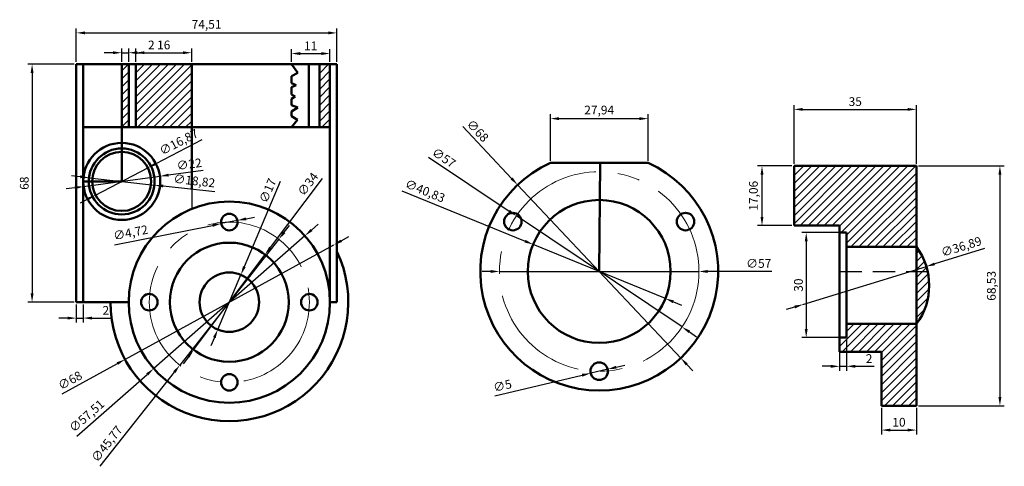
# Model space of a CAD drawing. Units: millimetres. Extents: x 1194 to 1920, y 1729 to 2086.
# Tile 2 of 5: x 1194 to 1475, y 1948 to 2076. Entities that reach past the tile are written whole.
import ezdxf

# ---------------------------------------------------------------- set-up
doc = ezdxf.new("R2010")
doc.units = ezdxf.units.MM
doc.linetypes.add('CENTER', pattern=[50.8, 31.75, -6.35, 6.35, -6.35])
doc.linetypes.add('HIDDEN', pattern=[9.525, 6.35, -3.175])
for name, color, linetype, lineweight in [('M-CNTR', 1, 'CENTER', 18), ('M-DIMS', 2, 'Continuous', 25), ('M-HATC', 8, 'Continuous', 18), ('M-HIDN', 4, 'HIDDEN', 25), ('M-OUTL', 7, 'Continuous', 50)]:
    doc.layers.add(name, color=color, linetype=linetype, lineweight=lineweight)
doc.styles.get("Standard").update_dxf_attribs({"font": 'arial.ttf'})
doc.dimstyles.new('ISO-25', dxfattribs={"dimtxt": 2.5, "dimasz": 2.5, "dimexe": 1.25, "dimexo": 0.625, "dimtad": 1, "dimtxsty": 'Standard', "dimcen": 2.5, "dimadec": 0, "dimazin": 0, "dimtfac": 1, "dimtmove": 0, "dimatfit": 3, "dimfxl": 1, "dimarcsym": 0})

# ---------------------------------------------------------------- blocks, each defined once
blk = doc.blocks.new('*U1')
blk.add_circle((0, 0), 2.36)
blk = doc.blocks.new('*U2')
at = {"layer": 'M-OUTL', "color": 0, "linetype": 'ByBlock', "lineweight": -2, "transparency": 16777216}
blk.add_blockref('*U1', (1253.67, 2017.83), dxfattribs=at)
for p, rotation in [((1230.79, 1994.94), 90), ((1276.56, 1994.94), 270), ((1253.67, 1972.06), 180)]:
    blk.add_blockref('*U1', p, dxfattribs=dict(at, rotation=rotation))
blk = doc.blocks.new('*U3')
blk.add_circle((0, 0), 2.5)
blk = doc.blocks.new('*U4')
at = {"layer": 'M-OUTL', "color": 0, "linetype": 'ByBlock', "lineweight": -2, "transparency": 16777216}
for p, rotation in [((1334.73, 2017.97), 240), ((1384.09, 2017.97), 119.9999999999999)]:
    blk.add_blockref('*U3', p, dxfattribs=dict(at, rotation=rotation))
blk.add_blockref('*U3', (1359.41, 1975.22), dxfattribs=at)
blk = doc.blocks.new('*D13')
at = {"layer": 'Defpoints', "color": 0, "transparency": 16777216}
for p in [(1283.49, 2011.28), (1223.86, 1978.6)]:
    blk.add_point(p, dxfattribs=at)
at = {"layer": 'M-DIMS', "color": 0, "lineweight": -2, "transparency": 16777216}
for p, q in [((1285.68, 2012.49), (1287.87, 2013.69)), ((1283.49, 2011.28), (1223.86, 1978.6)), ((1205.92, 1968.78), (1221.66, 1977.4))]:
    blk.add_line(p, q, dxfattribs=at)
at = {"layer": 'M-DIMS', "color": 0, "transparency": 16777216}
for points in [[(1285.48, 2012.85), (1285.88, 2012.12), (1283.49, 2011.28)], [(1221.46, 1977.77), (1221.86, 1977.04), (1223.86, 1978.6)]]:
    blk.add_solid(points, dxfattribs=at)
at = {"layer": 'M-DIMS', "color": 0, "transparency": 16777216, "insert": (1208.29, 1972.32), "char_height": 2.5, "attachment_point": 5, "rotation": 28.7233}
blk.add_mtext('∅68', dxfattribs=at)
blk = doc.blocks.new('*D14')
at = {"layer": 'Defpoints', "color": 0, "transparency": 16777216}
for p in [(1275.28, 2013.91), (1232.06, 1975.97)]:
    blk.add_point(p, dxfattribs=at)
at = {"layer": 'M-DIMS', "color": 0, "lineweight": -2, "transparency": 16777216}
for p, q in [((1277.16, 2015.56), (1279.04, 2017.21)), ((1275.28, 2013.91), (1232.06, 1975.97)), ((1210.06, 1956.65), (1230.19, 1974.33))]:
    blk.add_line(p, q, dxfattribs=at)
at = {"layer": 'M-DIMS', "color": 0, "transparency": 16777216}
for points in [[(1276.88, 2015.88), (1277.43, 2015.25), (1275.28, 2013.91)], [(1229.91, 1974.64), (1230.46, 1974.01), (1232.06, 1975.97)]]:
    blk.add_solid(points, dxfattribs=at)
at = {"layer": 'M-DIMS', "color": 0, "transparency": 16777216, "insert": (1213.11, 1962.22), "char_height": 2.5, "attachment_point": 5, "rotation": 41.2792}
blk.add_mtext('∅57,51', dxfattribs=at)
blk = doc.blocks.new('*D15')
at = {"layer": 'Defpoints', "color": 0, "transparency": 16777216}
for p in [(1267.82, 2012.93), (1239.52, 1976.96)]:
    blk.add_point(p, dxfattribs=at)
at = {"layer": 'M-DIMS', "color": 0, "lineweight": -2, "transparency": 16777216}
for p, q in [((1269.37, 2014.9), (1270.92, 2016.86)), ((1267.82, 2012.93), (1239.52, 1976.96)), ((1216.79, 1948.06), (1237.98, 1974.99))]:
    blk.add_line(p, q, dxfattribs=at)
at = {"layer": 'M-DIMS', "color": 0, "transparency": 16777216}
for points in [[(1269.04, 2015.15), (1269.7, 2014.64), (1267.82, 2012.93)], [(1237.65, 1975.25), (1238.3, 1974.73), (1239.52, 1976.96)]]:
    blk.add_solid(points, dxfattribs=at)
at = {"layer": 'M-DIMS', "color": 0, "transparency": 16777216, "insert": (1218.92, 1954.28), "char_height": 2.5, "attachment_point": 5, "rotation": 51.8058}
blk.add_mtext('∅45,77', dxfattribs=at)
blk = doc.blocks.new('*D16')
at = {"layer": 'Defpoints', "color": 0, "transparency": 16777216}
for p in [(1263.88, 2008.54), (1243.47, 1981.35)]:
    blk.add_point(p, dxfattribs=at)
at = {"layer": 'M-DIMS', "color": 0, "lineweight": -2, "transparency": 16777216}
for p, q in [((1280.22, 2030.3), (1265.38, 2010.54)), ((1243.47, 1981.35), (1263.88, 2008.54)), ((1241.96, 1979.35), (1240.46, 1977.35))]:
    blk.add_line(p, q, dxfattribs=at)
at = {"layer": 'M-DIMS', "color": 0, "transparency": 16777216}
for points in [[(1265.05, 2010.79), (1265.71, 2010.29), (1263.88, 2008.54)], [(1241.63, 1979.6), (1242.3, 1979.1), (1243.47, 1981.35)]]:
    blk.add_solid(points, dxfattribs=at)
at = {"layer": 'M-DIMS', "color": 0, "transparency": 16777216, "insert": (1276.38, 2028.47), "char_height": 2.5, "attachment_point": 5, "rotation": 53.1003}
blk.add_mtext('∅34', dxfattribs=at)
blk = doc.blocks.new('*D17')
at = {"layer": 'Defpoints', "color": 0, "transparency": 16777216}
for p in [(1256.98, 2002.77), (1250.36, 1987.11)]:
    blk.add_point(p, dxfattribs=at)
at = {"layer": 'M-DIMS', "color": 0, "lineweight": -2, "transparency": 16777216}
for p, q in [((1268.23, 2029.39), (1257.96, 2005.08)), ((1250.36, 1987.11), (1256.98, 2002.77)), ((1249.39, 1984.81), (1248.42, 1982.51))]:
    blk.add_line(p, q, dxfattribs=at)
at = {"layer": 'M-DIMS', "color": 0, "transparency": 16777216}
for points in [[(1257.57, 2005.24), (1258.34, 2004.91), (1256.98, 2002.77)], [(1249.01, 1984.97), (1249.77, 1984.65), (1250.36, 1987.11)]]:
    blk.add_solid(points, dxfattribs=at)
at = {"layer": 'M-DIMS', "color": 0, "transparency": 16777216, "insert": (1264.95, 2026.68), "char_height": 2.5, "attachment_point": 5, "rotation": 67.0856}
blk.add_mtext('∅17', dxfattribs=at)
blk = doc.blocks.new('*D18')
at = {"layer": 'Defpoints', "color": 0, "transparency": 16777216}
for p in [(1255.99, 2018.29), (1251.35, 2017.38)]:
    blk.add_point(p, dxfattribs=at)
at = {"layer": 'M-DIMS', "color": 0, "lineweight": -2, "transparency": 16777216}
for p, q in [((1255.99, 2018.29), (1251.35, 2017.38)), ((1258.44, 2018.77), (1260.9, 2019.25)), ((1220.8, 2011.37), (1248.9, 2016.89))]:
    blk.add_line(p, q, dxfattribs=at)
at = {"layer": 'M-DIMS', "color": 0, "transparency": 16777216}
for points in [[(1258.36, 2019.18), (1258.52, 2018.36), (1255.99, 2018.29)], [(1248.82, 2017.3), (1248.98, 2016.48), (1251.35, 2017.38)]]:
    blk.add_solid(points, dxfattribs=at)
at = {"layer": 'M-DIMS', "color": 0, "transparency": 16777216, "insert": (1225.51, 2014.5), "char_height": 2.5, "attachment_point": 5, "rotation": 11.1212}
blk.add_mtext('∅4,72', dxfattribs=at)
blk = doc.blocks.new('*D19')
at = {"layer": 'Defpoints', "color": 0, "transparency": 16777216}
for p in [(1233.82, 2030.92), (1212.02, 2027.97)]:
    blk.add_point(p, dxfattribs=at)
at = {"layer": 'M-DIMS', "color": 0, "lineweight": -2, "transparency": 16777216}
for p, q in [((1246.23, 2032.6), (1236.3, 2031.25)), ((1212.02, 2027.97), (1233.82, 2030.92)), ((1209.54, 2027.63), (1207.06, 2027.3))]:
    blk.add_line(p, q, dxfattribs=at)
at = {"layer": 'M-DIMS', "color": 0, "transparency": 16777216}
for points in [[(1236.24, 2031.67), (1236.35, 2030.84), (1233.82, 2030.92)], [(1209.48, 2028.05), (1209.6, 2027.22), (1212.02, 2027.97)]]:
    blk.add_solid(points, dxfattribs=at)
at = {"layer": 'M-DIMS', "color": 0, "transparency": 16777216, "insert": (1242.24, 2034.05), "char_height": 2.5, "attachment_point": 5, "rotation": 7.7042}
blk.add_mtext('∅22', dxfattribs=at)
blk = doc.blocks.new('*D20')
at = {"layer": 'Defpoints', "color": 0, "transparency": 16777216}
for p in [(1213.57, 2030.49), (1232.27, 2028.39)]:
    blk.add_point(p, dxfattribs=at)
at = {"layer": 'M-DIMS', "color": 0, "lineweight": -2, "transparency": 16777216}
for p, q in [((1211.08, 2030.77), (1208.6, 2031.05)), ((1213.57, 2030.49), (1232.27, 2028.39)), ((1249.54, 2026.46), (1234.75, 2028.12))]:
    blk.add_line(p, q, dxfattribs=at)
at = {"layer": 'M-DIMS', "color": 0, "transparency": 16777216}
for points in [[(1211.13, 2031.19), (1211.04, 2030.36), (1213.57, 2030.49)], [(1234.8, 2028.53), (1234.71, 2027.7), (1232.27, 2028.39)]]:
    blk.add_solid(points, dxfattribs=at)
at = {"layer": 'M-DIMS', "color": 0, "transparency": 16777216, "insert": (1243.63, 2029.3), "char_height": 2.5, "attachment_point": 5, "rotation": 353.5943}
blk.add_mtext('∅18,82', dxfattribs=at)
blk = doc.blocks.new('*D21')
at = {"layer": 'Defpoints', "color": 0, "transparency": 16777216}
for p in [(1230.41, 2033.33), (1215.43, 2025.56)]:
    blk.add_point(p, dxfattribs=at)
at = {"layer": 'M-DIMS', "color": 0, "lineweight": -2, "transparency": 16777216}
for p, q in [((1245.86, 2041.33), (1232.63, 2034.48)), ((1215.43, 2025.56), (1230.41, 2033.33)), ((1213.21, 2024.41), (1210.99, 2023.26))]:
    blk.add_line(p, q, dxfattribs=at)
at = {"layer": 'M-DIMS', "color": 0, "transparency": 16777216}
for points in [[(1232.44, 2034.85), (1232.82, 2034.11), (1230.41, 2033.33)], [(1213.02, 2024.78), (1213.4, 2024.04), (1215.43, 2025.56)]]:
    blk.add_solid(points, dxfattribs=at)
at = {"layer": 'M-DIMS', "color": 0, "transparency": 16777216, "insert": (1239.36, 2040.4), "char_height": 2.5, "attachment_point": 5, "rotation": 27.3904}
blk.add_mtext('∅16,87', dxfattribs=at)
blk = doc.blocks.new('*D22')
at = {"layer": 'Defpoints', "color": 0, "transparency": 16777216}
for p in [(1209.92, 2062.94), (1197.29, 1994.94), (1209.92, 1994.94)]:
    blk.add_point(p, dxfattribs=at)
at = {"layer": 'M-DIMS', "color": 0, "lineweight": -2, "transparency": 16777216}
for p, q in [((1209.29, 2062.94), (1196.04, 2062.94)), ((1197.29, 2060.44), (1197.29, 1997.44)), ((1209.29, 1994.94), (1196.04, 1994.94))]:
    blk.add_line(p, q, dxfattribs=at)
at = {"layer": 'M-DIMS', "color": 0, "transparency": 16777216}
for points in [[(1196.87, 2060.44), (1197.7, 2060.44), (1197.29, 2062.94)], [(1196.87, 1997.44), (1197.7, 1997.44), (1197.29, 1994.94)]]:
    blk.add_solid(points, dxfattribs=at)
at = {"layer": 'M-DIMS', "color": 0, "transparency": 16777216, "insert": (1195.38, 2028.94), "char_height": 2.5, "attachment_point": 5, "rotation": 90}
blk.add_mtext('68', dxfattribs=at)
blk = doc.blocks.new('*D23')
at = {"layer": 'Defpoints', "color": 0, "transparency": 16777216}
for p in [(1284.43, 2071.87), (1209.92, 2062.94), (1284.43, 2062.94)]:
    blk.add_point(p, dxfattribs=at)
at = {"layer": 'M-DIMS', "color": 0, "lineweight": -2, "transparency": 16777216}
for p, q in [((1209.92, 2063.57), (1209.92, 2073.12)), ((1212.42, 2071.87), (1281.93, 2071.87)), ((1284.43, 2063.57), (1284.43, 2073.12))]:
    blk.add_line(p, q, dxfattribs=at)
at = {"layer": 'M-DIMS', "color": 0, "transparency": 16777216}
for points in [[(1212.42, 2072.29), (1212.42, 2071.46), (1209.92, 2071.87)], [(1281.93, 2072.29), (1281.93, 2071.46), (1284.43, 2071.87)]]:
    blk.add_solid(points, dxfattribs=at)
at = {"layer": 'M-DIMS', "color": 0, "transparency": 16777216, "insert": (1247.17, 2074), "char_height": 2.5, "attachment_point": 5}
blk.add_mtext('74,51', dxfattribs=at)
blk = doc.blocks.new('*D24')
at = {"layer": 'Defpoints', "color": 0, "transparency": 16777216}
for p in [(1224.92, 2066.21), (1222.92, 2062.94), (1224.92, 2062.94)]:
    blk.add_point(p, dxfattribs=at)
at = {"layer": 'M-DIMS', "color": 0, "lineweight": -2, "transparency": 16777216}
for p, q in [((1220.42, 2066.21), (1217.92, 2066.21)), ((1222.92, 2063.57), (1222.92, 2067.46)), ((1222.92, 2066.21), (1224.92, 2066.21)), ((1224.92, 2063.57), (1224.92, 2067.46)), ((1227.42, 2066.21), (1232.82, 2066.21))]:
    blk.add_line(p, q, dxfattribs=at)
at = {"layer": 'M-DIMS', "color": 0, "transparency": 16777216}
for points in [[(1220.42, 2066.63), (1220.42, 2065.8), (1222.92, 2066.21)], [(1227.42, 2066.63), (1227.42, 2065.8), (1224.92, 2066.21)]]:
    blk.add_solid(points, dxfattribs=at)
at = {"layer": 'M-DIMS', "color": 0, "transparency": 16777216, "insert": (1231.37, 2068.09), "char_height": 2.5, "attachment_point": 5}
blk.add_mtext('2', dxfattribs=at)
blk = doc.blocks.new('*D25')
at = {"layer": 'Defpoints', "color": 0, "transparency": 16777216}
for p in [(1242.92, 2066.21), (1226.92, 2062.94), (1242.92, 2062.94)]:
    blk.add_point(p, dxfattribs=at)
at = {"layer": 'M-DIMS', "color": 0, "lineweight": -2, "transparency": 16777216}
for p, q in [((1226.92, 2063.57), (1226.92, 2067.46)), ((1229.42, 2066.21), (1240.42, 2066.21)), ((1242.92, 2063.57), (1242.92, 2067.46))]:
    blk.add_line(p, q, dxfattribs=at)
at = {"layer": 'M-DIMS', "color": 0, "transparency": 16777216}
for points in [[(1229.42, 2066.63), (1229.42, 2065.8), (1226.92, 2066.21)], [(1240.42, 2066.63), (1240.42, 2065.8), (1242.92, 2066.21)]]:
    blk.add_solid(points, dxfattribs=at)
at = {"layer": 'M-DIMS', "color": 0, "transparency": 16777216, "insert": (1234.92, 2068.11), "char_height": 2.5, "attachment_point": 5}
blk.add_mtext('16', dxfattribs=at)
blk = doc.blocks.new('*D26')
at = {"layer": 'Defpoints', "color": 0, "transparency": 16777216}
for p in [(1282.43, 2065.97), (1271.43, 2062.94), (1282.43, 2062.94)]:
    blk.add_point(p, dxfattribs=at)
at = {"layer": 'M-DIMS', "color": 0, "lineweight": -2, "transparency": 16777216}
for p, q in [((1271.43, 2063.57), (1271.43, 2067.22)), ((1282.43, 2063.57), (1282.43, 2067.22)), ((1273.93, 2065.97), (1279.93, 2065.97))]:
    blk.add_line(p, q, dxfattribs=at)
at = {"layer": 'M-DIMS', "color": 0, "transparency": 16777216}
for points in [[(1273.93, 2066.39), (1273.93, 2065.55), (1271.43, 2065.97)], [(1279.93, 2066.39), (1279.93, 2065.55), (1282.43, 2065.97)]]:
    blk.add_solid(points, dxfattribs=at)
at = {"layer": 'M-DIMS', "color": 0, "transparency": 16777216, "insert": (1276.93, 2067.85), "char_height": 2.5, "attachment_point": 5}
blk.add_mtext('11', dxfattribs=at)
blk = doc.blocks.new('*D27')
at = {"layer": 'Defpoints', "color": 0, "transparency": 16777216}
for p in [(1209.92, 1994.94), (1211.92, 1994.94), (1211.92, 1990.4)]:
    blk.add_point(p, dxfattribs=at)
at = {"layer": 'M-DIMS', "color": 0, "lineweight": -2, "transparency": 16777216}
for p, q in [((1209.92, 1994.32), (1209.92, 1989.15)), ((1211.92, 1994.32), (1211.92, 1989.15)), ((1207.42, 1990.4), (1204.92, 1990.4)), ((1209.92, 1990.4), (1211.92, 1990.4)), ((1214.42, 1990.4), (1219.82, 1990.4))]:
    blk.add_line(p, q, dxfattribs=at)
at = {"layer": 'M-DIMS', "color": 0, "transparency": 16777216}
for points in [[(1207.42, 1990.82), (1207.42, 1989.98), (1209.92, 1990.4)], [(1214.42, 1990.82), (1214.42, 1989.98), (1211.92, 1990.4)]]:
    blk.add_solid(points, dxfattribs=at)
at = {"layer": 'M-DIMS', "color": 0, "transparency": 16777216, "insert": (1218.37, 1992.28), "char_height": 2.5, "attachment_point": 5}
blk.add_mtext('2', dxfattribs=at)
blk = doc.blocks.new('*D28')
at = {"layer": 'Defpoints', "color": 0, "transparency": 16777216}
for p in [(1336.09, 2028.46), (1382.73, 1978.98)]:
    blk.add_point(p, dxfattribs=at)
at = {"layer": 'M-DIMS', "color": 0, "lineweight": -2, "transparency": 16777216}
for p, q in [((1320.41, 2045.1), (1334.38, 2030.28)), ((1382.73, 1978.98), (1336.09, 2028.46)), ((1384.45, 1977.16), (1386.16, 1975.34))]:
    blk.add_line(p, q, dxfattribs=at)
at = {"layer": 'M-DIMS', "color": 0, "transparency": 16777216}
for points in [[(1334.68, 2030.57), (1334.07, 2029.99), (1336.09, 2028.46)], [(1384.75, 1977.44), (1384.15, 1976.87), (1382.73, 1978.98)]]:
    blk.add_solid(points, dxfattribs=at)
at = {"layer": 'M-DIMS', "color": 0, "transparency": 16777216, "insert": (1324.44, 2043.7), "char_height": 2.5, "attachment_point": 5, "rotation": 313.3071}
blk.add_mtext('∅68', dxfattribs=at)
blk = doc.blocks.new('*D29')
at = {"layer": 'Defpoints', "color": 0, "transparency": 16777216}
for p in [(1335.73, 2019.57), (1383.1, 1987.87)]:
    blk.add_point(p, dxfattribs=at)
at = {"layer": 'M-DIMS', "color": 0, "lineweight": -2, "transparency": 16777216}
for p, q in [((1310.6, 2036.39), (1333.65, 2020.96)), ((1383.1, 1987.87), (1335.73, 2019.57)), ((1385.18, 1986.48), (1387.25, 1985.09))]:
    blk.add_line(p, q, dxfattribs=at)
at = {"layer": 'M-DIMS', "color": 0, "transparency": 16777216}
for points in [[(1333.88, 2021.31), (1333.42, 2020.62), (1335.73, 2019.57)], [(1385.41, 1986.82), (1384.94, 1986.13), (1383.1, 1987.87)]]:
    blk.add_solid(points, dxfattribs=at)
at = {"layer": 'M-DIMS', "color": 0, "transparency": 16777216, "insert": (1314.83, 2035.93), "char_height": 2.5, "attachment_point": 5, "rotation": 326.2049}
blk.add_mtext('∅57', dxfattribs=at)
blk = doc.blocks.new('*D30')
at = {"layer": 'Defpoints', "color": 0, "transparency": 16777216}
for p in [(1340.51, 2011.44), (1378.32, 1996)]:
    blk.add_point(p, dxfattribs=at)
at = {"layer": 'M-DIMS', "color": 0, "lineweight": -2, "transparency": 16777216}
for p, q in [((1302.95, 2026.77), (1338.2, 2012.38)), ((1378.32, 1996), (1340.51, 2011.44)), ((1380.63, 1995.06), (1382.94, 1994.11))]:
    blk.add_line(p, q, dxfattribs=at)
at = {"layer": 'M-DIMS', "color": 0, "transparency": 16777216}
for points in [[(1338.35, 2012.77), (1338.04, 2012), (1340.51, 2011.44)], [(1380.79, 1995.44), (1380.47, 1994.67), (1378.32, 1996)]]:
    blk.add_solid(points, dxfattribs=at)
at = {"layer": 'M-DIMS', "color": 0, "transparency": 16777216, "insert": (1309.51, 2026.44), "char_height": 2.5, "attachment_point": 5, "rotation": 337.7892}
blk.add_mtext('∅40,83', dxfattribs=at)
blk = doc.blocks.new('*D31')
at = {"layer": 'Defpoints', "color": 0, "transparency": 16777216}
for p in [(1356.98, 1974.65), (1361.85, 1975.79)]:
    blk.add_point(p, dxfattribs=at)
at = {"layer": 'M-DIMS', "color": 0, "lineweight": -2, "transparency": 16777216}
for p, q in [((1364.28, 1976.36), (1366.72, 1976.93)), ((1329.53, 1968.22), (1354.55, 1974.08)), ((1361.85, 1975.79), (1356.98, 1974.65))]:
    blk.add_line(p, q, dxfattribs=at)
at = {"layer": 'M-DIMS', "color": 0, "transparency": 16777216}
for points in [[(1364.19, 1976.77), (1364.38, 1975.95), (1361.85, 1975.79)], [(1354.45, 1974.48), (1354.64, 1973.67), (1356.98, 1974.65)]]:
    blk.add_solid(points, dxfattribs=at)
at = {"layer": 'M-DIMS', "color": 0, "transparency": 16777216, "insert": (1331.82, 1970.78), "char_height": 2.5, "attachment_point": 5, "rotation": 13.1908}
blk.add_mtext('∅5', dxfattribs=at)
blk = doc.blocks.new('*D32')
at = {"layer": 'Defpoints', "color": 0, "transparency": 16777216}
for p in [(1373.38, 2047.38), (1345.45, 2034.72), (1373.38, 2034.72)]:
    blk.add_point(p, dxfattribs=at)
at = {"layer": 'M-DIMS', "color": 0, "lineweight": -2, "transparency": 16777216}
for p, q in [((1345.45, 2035.34), (1345.45, 2048.63)), ((1347.95, 2047.38), (1370.88, 2047.38)), ((1373.38, 2035.34), (1373.38, 2048.63))]:
    blk.add_line(p, q, dxfattribs=at)
at = {"layer": 'M-DIMS', "color": 0, "transparency": 16777216}
for points in [[(1347.95, 2047.8), (1347.95, 2046.96), (1345.45, 2047.38)], [(1370.88, 2047.8), (1370.88, 2046.96), (1373.38, 2047.38)]]:
    blk.add_solid(points, dxfattribs=at)
at = {"layer": 'M-DIMS', "color": 0, "transparency": 16777216, "insert": (1359.41, 2049.51), "char_height": 2.5, "attachment_point": 5}
blk.add_mtext('27,94', dxfattribs=at)
blk = doc.blocks.new('*D33')
at = {"layer": 'Defpoints', "color": 0, "transparency": 16777216}
for p in [(1450.11, 2050.02), (1415.11, 2033.89), (1450.11, 2033.89)]:
    blk.add_point(p, dxfattribs=at)
at = {"layer": 'M-DIMS', "color": 0, "lineweight": -2, "transparency": 16777216}
for p, q in [((1415.11, 2034.51), (1415.11, 2051.27)), ((1417.61, 2050.02), (1447.61, 2050.02)), ((1450.11, 2034.51), (1450.11, 2051.27))]:
    blk.add_line(p, q, dxfattribs=at)
at = {"layer": 'M-DIMS', "color": 0, "transparency": 16777216}
for points in [[(1417.61, 2050.44), (1417.61, 2049.61), (1415.11, 2050.02)], [(1447.61, 2050.44), (1447.61, 2049.61), (1450.11, 2050.02)]]:
    blk.add_solid(points, dxfattribs=at)
at = {"layer": 'M-DIMS', "color": 0, "transparency": 16777216, "insert": (1432.61, 2051.92), "char_height": 2.5, "attachment_point": 5}
blk.add_mtext('35', dxfattribs=at)
blk = doc.blocks.new('*D34')
at = {"layer": 'Defpoints', "color": 0, "transparency": 16777216}
for p in [(1415.11, 2033.89), (1405.95, 2016.82), (1415.11, 2016.82)]:
    blk.add_point(p, dxfattribs=at)
at = {"layer": 'M-DIMS', "color": 0, "lineweight": -2, "transparency": 16777216}
for p, q in [((1414.48, 2033.89), (1404.7, 2033.89)), ((1405.95, 2031.39), (1405.95, 2019.32)), ((1414.48, 2016.82), (1404.7, 2016.82))]:
    blk.add_line(p, q, dxfattribs=at)
at = {"layer": 'M-DIMS', "color": 0, "transparency": 16777216}
for points in [[(1405.54, 2031.39), (1406.37, 2031.39), (1405.95, 2033.89)], [(1405.54, 2019.32), (1406.37, 2019.32), (1405.95, 2016.82)]]:
    blk.add_solid(points, dxfattribs=at)
at = {"layer": 'M-DIMS', "color": 0, "transparency": 16777216, "insert": (1403.82, 2025.36), "char_height": 2.5, "attachment_point": 5, "rotation": 90}
blk.add_mtext('17,06', dxfattribs=at)
blk = doc.blocks.new('*D35')
at = {"layer": 'Defpoints', "color": 0, "transparency": 16777216}
for p in [(1450.11, 2033.89), (1450.11, 1965.36), (1473.97, 1965.36)]:
    blk.add_point(p, dxfattribs=at)
at = {"layer": 'M-DIMS', "color": 0, "lineweight": -2, "transparency": 16777216}
for p, q in [((1450.73, 2033.89), (1475.22, 2033.89)), ((1473.97, 2031.39), (1473.97, 1967.86)), ((1450.73, 1965.36), (1475.22, 1965.36))]:
    blk.add_line(p, q, dxfattribs=at)
at = {"layer": 'M-DIMS', "color": 0, "transparency": 16777216}
for points in [[(1473.55, 2031.39), (1474.39, 2031.39), (1473.97, 2033.89)], [(1473.55, 1967.86), (1474.39, 1967.86), (1473.97, 1965.36)]]:
    blk.add_solid(points, dxfattribs=at)
at = {"layer": 'M-DIMS', "color": 0, "transparency": 16777216, "insert": (1471.84, 1999.62), "char_height": 2.5, "attachment_point": 5, "rotation": 90}
blk.add_mtext('68,53', dxfattribs=at)
blk = doc.blocks.new('*D36')
at = {"layer": 'Defpoints', "color": 0, "transparency": 16777216}
for p in [(1430.12, 2014.82), (1418.59, 1984.82), (1430.12, 1984.82)]:
    blk.add_point(p, dxfattribs=at)
at = {"layer": 'M-DIMS', "color": 0, "lineweight": -2, "transparency": 16777216}
for p, q in [((1429.5, 2014.82), (1417.34, 2014.82)), ((1418.59, 2012.32), (1418.59, 1987.32)), ((1429.5, 1984.82), (1417.34, 1984.82))]:
    blk.add_line(p, q, dxfattribs=at)
at = {"layer": 'M-DIMS', "color": 0, "transparency": 16777216}
for points in [[(1418.18, 2012.32), (1419.01, 2012.32), (1418.59, 2014.82)], [(1418.18, 1987.32), (1419.01, 1987.32), (1418.59, 1984.82)]]:
    blk.add_solid(points, dxfattribs=at)
at = {"layer": 'M-DIMS', "color": 0, "transparency": 16777216, "insert": (1416.69, 1999.82), "char_height": 2.5, "attachment_point": 5, "rotation": 90}
blk.add_mtext('30', dxfattribs=at)
blk = doc.blocks.new('*D37')
at = {"layer": 'Defpoints', "color": 0, "transparency": 16777216}
for p in [(1428.12, 1984.82), (1430.12, 1984.82), (1430.12, 1976.62)]:
    blk.add_point(p, dxfattribs=at)
at = {"layer": 'M-DIMS', "color": 0, "lineweight": -2, "transparency": 16777216}
for p, q in [((1428.12, 1984.2), (1428.12, 1975.37)), ((1430.12, 1984.2), (1430.12, 1975.37)), ((1425.62, 1976.62), (1423.12, 1976.62)), ((1428.12, 1976.62), (1430.12, 1976.62)), ((1432.62, 1976.62), (1438.03, 1976.62))]:
    blk.add_line(p, q, dxfattribs=at)
at = {"layer": 'M-DIMS', "color": 0, "transparency": 16777216}
for points in [[(1425.62, 1977.04), (1425.62, 1976.2), (1428.12, 1976.62)], [(1432.62, 1977.04), (1432.62, 1976.2), (1430.12, 1976.62)]]:
    blk.add_solid(points, dxfattribs=at)
at = {"layer": 'M-DIMS', "color": 0, "transparency": 16777216, "insert": (1436.57, 1978.5), "char_height": 2.5, "attachment_point": 5}
blk.add_mtext('2', dxfattribs=at)
blk = doc.blocks.new('*D38')
at = {"layer": 'Defpoints', "color": 0, "transparency": 16777216}
for p in [(1452.93, 2005.14), (1417.67, 1994.3)]:
    blk.add_point(p, dxfattribs=at)
at = {"layer": 'M-DIMS', "color": 0, "lineweight": -2, "transparency": 16777216}
for p, q in [((1469.57, 2010.26), (1455.32, 2005.87)), ((1417.67, 1994.3), (1452.93, 2005.14)), ((1415.28, 1993.56), (1412.89, 1992.83))]:
    blk.add_line(p, q, dxfattribs=at)
at = {"layer": 'M-DIMS', "color": 0, "transparency": 16777216}
for points in [[(1455.2, 2006.27), (1455.44, 2005.48), (1452.93, 2005.14)], [(1415.16, 1993.96), (1415.4, 1993.17), (1417.67, 1994.3)]]:
    blk.add_solid(points, dxfattribs=at)
at = {"layer": 'M-DIMS', "color": 0, "transparency": 16777216, "insert": (1463.01, 2010.51), "char_height": 2.5, "attachment_point": 5, "rotation": 17.0881}
blk.add_mtext('∅36,89', dxfattribs=at)
blk = doc.blocks.new('*D39')
at = {"layer": 'Defpoints', "color": 0, "transparency": 16777216}
for p in [(1440.11, 1965.36), (1450.11, 1965.36), (1450.11, 1958.41)]:
    blk.add_point(p, dxfattribs=at)
at = {"layer": 'M-DIMS', "color": 0, "lineweight": -2, "transparency": 16777216}
for p, q in [((1440.11, 1964.73), (1440.11, 1957.16)), ((1450.11, 1964.73), (1450.11, 1957.16)), ((1442.61, 1958.41), (1447.61, 1958.41))]:
    blk.add_line(p, q, dxfattribs=at)
at = {"layer": 'M-DIMS', "color": 0, "transparency": 16777216}
for points in [[(1442.61, 1958.83), (1442.61, 1958), (1440.11, 1958.41)], [(1447.61, 1958.83), (1447.61, 1958), (1450.11, 1958.41)]]:
    blk.add_solid(points, dxfattribs=at)
at = {"layer": 'M-DIMS', "color": 0, "transparency": 16777216, "insert": (1445.11, 1960.32), "char_height": 2.5, "attachment_point": 5}
blk.add_mtext('10', dxfattribs=at)
blk = doc.blocks.new('*D144')
at = {"layer": 'Defpoints', "color": 0, "transparency": 16777216}
for p in [(1330.91, 2003.72), (1387.91, 2003.72)]:
    blk.add_point(p, dxfattribs=at)
at = {"layer": 'M-DIMS', "color": 0, "lineweight": -2, "transparency": 16777216}
for p, q in [((1328.41, 2003.72), (1325.91, 2003.72)), ((1330.91, 2003.72), (1387.91, 2003.72)), ((1408.79, 2003.72), (1390.41, 2003.72))]:
    blk.add_line(p, q, dxfattribs=at)
at = {"layer": 'M-DIMS', "color": 0, "transparency": 16777216}
for points in [[(1328.41, 2004.14), (1328.41, 2003.3), (1330.91, 2003.72)], [(1390.41, 2004.14), (1390.41, 2003.3), (1387.91, 2003.72)]]:
    blk.add_solid(points, dxfattribs=at)
at = {"layer": 'M-DIMS', "color": 0, "transparency": 16777216, "insert": (1405.01, 2005.69), "char_height": 2.5, "attachment_point": 5, "rotation": 359.9991}
blk.add_mtext('∅57', dxfattribs=at)

msp = doc.modelspace()

# ---------------------------------------------------------------- hatches: boundary and pattern name
at = {"layer": 'M-HATC'}
h = msp.add_hatch(dxfattribs=at)
h.set_pattern_fill('ANSI31', color=256, scale=0.51)
h.paths.add_polyline_path([(1282.426, 2062.9441), (1279.426, 2062.9441), (1279.426, 2044.9441), (1282.426, 2044.9441)])
h.paths.add_polyline_path([(1242.9188, 2062.9441), (1226.9188, 2062.9441), (1226.9188, 2044.9441), (1242.9188, 2044.9441)])
h.paths.add_polyline_path([(1224.9188, 2062.9441), (1222.9188, 2062.9441), (1222.9188, 2044.9441), (1224.9188, 2044.9441)])
h = msp.add_hatch(dxfattribs=at)
h.set_pattern_fill('ANSI31', color=256, scale=0.51)
h.paths.add_polyline_path([(1450.1079, 2033.8878), (1415.1079, 2033.8878), (1415.1079, 2016.8229), (1428.1211, 2016.8229), (1428.1211, 2014.8229), (1430.1211, 2014.8229), (1430.1211, 2010.7194), (1450.1079, 2010.7194)])
h.paths.add_polyline_path([(1450.1079, 1988.7194), (1430.1211, 1988.7194), (1430.1211, 1984.8229), (1428.1211, 1984.8229), (1428.1211, 1980.797), (1440.1079, 1980.797), (1440.1079, 1965.3573), (1450.1079, 1965.3573)])
h.paths.add_polyline_path([(1453.3077, 2003.7194), (1450.1079, 2003.7194), (1450.1079, 1988.7194, 0.21771974)])
h.paths.add_polyline_path([(1450.1079, 2010.7194), (1450.1079, 2003.7194), (1453.3077, 2003.7194, 0.10547185)])

# ---------------------------------------------------------------- linework, layer by layer
at = {"layer": 'M-CNTR'}
for centre, radius in [((1359.4131, 2003.7194), 28.5), ((1253.6724, 1994.9441), 22.8866)]:
    msp.add_circle(centre, radius, dxfattribs=at)
at = {"layer": 'M-HIDN'}
for p, q in [((1242.9188, 2027.1988), (1242.9756, 2021.634)), ((1428.1211, 2003.7194), (1453.3077, 2003.7194))]:
    msp.add_line(p, q, dxfattribs=at)
at = {"layer": 'M-OUTL'}
for p, q in [((1209.9188, 1994.9441), (1209.9188, 2062.9441)), ((1209.9188, 2062.9441), (1284.426, 2062.9441)), ((1211.9188, 1994.9441), (1211.9188, 2062.9441)), ((1211.9188, 2062.9441), (1211.9188, 2057.9441)), ((1211.9188, 2062.9441), (1211.9188, 2062.9441)), ((1211.9188, 2062.9441), (1211.9188, 2044.9441)), ((1222.9188, 2029.4441), (1222.9188, 2062.9441)), ((1222.9188, 2062.9441), (1224.9188, 2062.9441)), ((1224.9188, 2062.9441), (1224.9188, 2044.9441)), ((1226.9188, 2044.9441), (1226.9188, 2062.9441)), ((1242.9188, 2062.9441), (1242.9188, 2027.1988)), ((1273.2203, 2060.4978), (1271.426, 2062.9441)), ((1271.426, 2062.9441), (1276.426, 2062.9441)), ((1271.426, 2059.5185), (1273.2203, 2060.4978)), ((1276.426, 2044.9441), (1276.426, 2062.9441)), ((1282.426, 2062.9441), (1279.426, 2062.9441)), ((1279.426, 2062.9441), (1279.426, 2044.9441)), ((1282.426, 1994.9441), (1282.426, 2062.9441)), ((1284.426, 1994.9441), (1284.426, 2062.9441)), ((1271.426, 2059.5185), (1271.426, 2057.549)), ((1272.7395, 2056.8975), (1271.426, 2057.549)), ((1271.426, 2056.381), (1272.7395, 2056.8975)), ((1271.426, 2056.381), (1271.426, 2054.3136)), ((1272.5375, 2053.749), (1271.426, 2054.3136)), ((1271.426, 2053.0011), (1272.5375, 2053.749)), ((1271.426, 2053.0011), (1271.426, 2051.2096)), ((1273.2878, 2050.5195), (1271.426, 2051.2096)), ((1271.426, 2049.4035), (1273.2878, 2050.5195)), ((1271.426, 2049.4035), (1271.426, 2048.1286)), ((1273.1724, 2047.0017), (1271.426, 2048.1286)), ((1271.426, 2044.9441), (1273.1724, 2047.0017)), ((1273.1724, 2047.0017), (1271.426, 2044.9441)), ((1271.426, 2044.9441), (1273.1724, 2047.0017)), ((1211.9188, 2044.9441), (1282.426, 2044.9441)), ((1276.426, 2044.9441), (1271.426, 2044.9441)), ((1359.747, 2034.7178), (1345.4452, 2034.7178)), ((1359.4131, 2003.7194), (1359.7175, 2034.7178)), ((1359.7175, 2034.7178), (1373.381, 2034.7178)), ((1415.1079, 2033.8878), (1450.1079, 2033.8878)), ((1415.1079, 2033.8878), (1415.1079, 2016.8229)), ((1450.1079, 2033.8878), (1450.1079, 1965.3573)), ((1211.9188, 1994.9441), (1211.9188, 2029.4441)), ((1211.9188, 2029.4441), (1222.9188, 2029.4441)), ((1428.1211, 2016.8229), (1415.1079, 2016.8229)), ((1428.1211, 1980.797), (1428.1211, 2016.8229)), ((1428.1211, 2016.8229), (1428.1211, 2014.8229)), ((1428.1211, 2014.8229), (1430.1211, 2014.8229)), ((1430.1211, 2014.8229), (1430.1211, 1984.8229)), ((1450.1079, 2010.7194), (1430.1211, 2010.7194)), ((1428.1211, 2003.7194), (1428.1211, 1988.7194)), ((1224.9188, 1994.9441), (1209.9188, 1994.9441)), ((1209.9188, 1994.9441), (1211.9188, 1994.9441)), ((1282.426, 1994.9441), (1284.426, 1994.9441)), ((1430.1211, 1988.7194), (1450.1079, 1988.7194)), ((1430.1211, 1984.8229), (1428.1211, 1984.8229)), ((1440.1079, 1980.797), (1428.1211, 1980.797)), ((1440.1079, 1965.3573), (1440.1079, 1980.797)), ((1450.1079, 1965.3573), (1440.1079, 1965.3573))]:
    msp.add_line(p, q, dxfattribs=at)
for centre, radius in [((1222.9188, 2029.4441), 11), ((1222.9188, 2029.4441), 9.4104), ((1222.9188, 2029.4441), 8.4372), ((1359.4131, 2003.7194), 20.4175), ((1253.6724, 1994.9441), 28.7536), ((1253.6724, 1994.9441), 17), ((1253.6724, 1994.9441), 8.5)]:
    msp.add_circle(centre, radius, dxfattribs=at)
for centre, radius, start, end in [((1359.4131, 2003.7194), 34, 114.256353, 65.743647), ((1435.3003, 1999.7194), 18.4463, 323.392854, 36.607146), ((1253.6724, 1994.9441), 34, 180, 25.241588)]:
    msp.add_arc(centre, radius, start, end, dxfattribs=at)

# ---------------------------------------------------------------- block references
for name in ['*U4', '*U2']:
    msp.add_blockref(name, (0, 0), dxfattribs=at)

# ---------------------------------------------------------------- dimensions: what is measured, and where the dimension line sits
at = {"layer": 'M-DIMS'}
for base, p1, p2, picture, middle in [((1284.426, 2071.8742), (1209.9188, 2062.9441), (1284.426, 2062.9441), '*D23', (1247.1724, 2074.0016)), ((1224.9188, 2066.2131), (1222.9188, 2062.9441), (1224.9188, 2062.9441), '*D24', (1231.3718, 2068.0932)), ((1242.9188, 2066.2131), (1226.9188, 2062.9441), (1242.9188, 2062.9441), '*D25', (1234.9188, 2068.1146)), ((1282.426, 2065.969), (1271.426, 2062.9441), (1282.426, 2062.9441), '*D26', (1276.926, 2067.8491)), ((1450.1079, 2050.0221), (1415.1079, 2033.8878), (1450.1079, 2033.8878), '*D33', (1432.6079, 2051.9243)), ((1373.381, 2047.3812), (1345.4452, 2034.7178), (1373.381, 2034.7178), '*D32', (1359.4131, 2049.5085)), ((1211.9188, 1990.4009), (1209.9188, 1994.9441), (1211.9188, 1994.9441), '*D27', (1218.3718, 1992.281)), ((1430.1211, 1976.6197), (1428.1211, 1984.8229), (1430.1211, 1984.8229), '*D37', (1436.5741, 1978.4998)), ((1450.1079, 1958.4145), (1440.1079, 1965.3573), (1450.1079, 1965.3573), '*D39', (1445.1079, 1960.3159))]:
    dim = msp.add_linear_dim(base=base, p1=p1, p2=p2, dimstyle='ISO-25', override={"dimclrd": 0, "dimclre": 0, "dimclrt": 0}, dxfattribs=at)
    dim.commit()
    dim.dimension.update_dxf_attribs({"geometry": picture, "text_midpoint": middle})
for base, p1, p2, picture, middle in [((1197.2862, 1994.9441), (1209.9188, 2062.9441), (1209.9188, 1994.9441), '*D22', (1195.3848, 2028.9441)), ((1405.9523, 2016.8229), (1415.1079, 2033.8878), (1415.1079, 2016.8229), '*D34', (1403.8249, 2025.3553)), ((1473.9709, 1965.3573), (1450.1079, 2033.8878), (1450.1079, 1965.3573), '*D35', (1471.8435, 1999.6226)), ((1418.5922, 1984.8229), (1430.1211, 2014.8229), (1430.1211, 1984.8229), '*D36', (1416.6899, 1999.8229))]:
    dim = msp.add_linear_dim(base=base, p1=p1, p2=p2, angle=90, dimstyle='ISO-25', override={"dimclrd": 0, "dimclre": 0, "dimclrt": 0}, dxfattribs=at)
    dim.commit()
    dim.dimension.update_dxf_attribs({"geometry": picture, "text_midpoint": middle})
for p1, p2, override, picture, middle in [((1382.734, 1978.9781), (1336.0922, 2028.4608), {"dimclrd": 0, "dimclre": 0, "dimclrt": 0}, '*D28', (1323.0027, 2042.3476)), ((1383.0975, 1987.867), (1335.7287, 2019.5718), {"dimclrd": 0, "dimclre": 0, "dimclrt": 0}, '*D29', (1313.7329, 2034.294)), ((1243.4654, 1981.3494), (1263.8795, 2008.5388), {"dimclrd": 0, "dimclre": 0, "dimclrt": 0}, '*D16', (1277.9543, 2027.285)), ((1250.3629, 1987.1149), (1256.982, 2002.7734), {"dimclrd": 0, "dimclre": 0, "dimclrt": 0}, '*D17', (1266.7628, 2025.9118)), ((1378.315616, 1996.001294), (1340.510613, 2011.437572), {"dimclrd": 0, "dimclre": 0, "dimclrt": 0}, '*D30', (1308.694991, 2024.428308)), ((1255.9903, 2018.2864), (1251.3546, 2017.3751), {"dimclrd": 0, "dimclre": 0, "dimclrt": 0}, '*D18', (1225.9238, 2012.376)), ((1275.2809, 2013.9137), (1232.064, 1975.9746), {"dimclrd": 0, "dimclre": 0, "dimclrt": 0}, '*D14', (1214.5359, 1960.5871)), ((1267.8239, 2012.9312), (1239.521, 1976.9571), {"dimclrd": 0, "dimclre": 0, "dimclrt": 0}, '*D15', (1220.6225, 1952.9364)), ((1283.4888, 2011.2838), (1223.8561, 1978.6044), {"dimclrd": 0, "dimclre": 0, "dimclrt": 0}, '*D13', (1209.2347, 1970.5918)), ((1330.9131, 2003.7199), (1387.9131, 2003.719), {"dimdec": 0, "dimlfac": 1, "dimrnd": 0, "dimzin": 0, "dimdsep": 46, "dimlunit": 2}, '*D144', (1405.0131, 2003.7187)), ((1361.8472, 1975.7899), (1356.9791, 1974.6489), {"dimclrd": 0, "dimclre": 0, "dimclrt": 0}, '*D31', (1332.2725, 1968.8583))]:
    dim = msp.add_diameter_dim_2p(p1=p1, p2=p2, dimstyle='ISO-25', override=override, dxfattribs=at)
    dim.commit()
    dim.dimension.update_dxf_attribs({"geometry": picture, "text_midpoint": middle, "dimtype": 163})
for p1, p2, picture, middle in [((1215.4275, 2025.5626), (1230.4101, 2033.3257), '*D21', (1239.3597, 2040.4049)), ((1212.0181, 2027.9695), (1233.8195, 2030.9188), '*D19', (1242.2389, 2034.0471)), ((1213.5672, 2030.494), (1232.2705, 2028.3942), '*D20', (1243.6328, 2029.3005)), ((1417.6683, 1994.2991), (1452.9323, 2005.1397), '*D38', (1463.0061, 2010.505))]:
    dim = msp.add_diameter_dim_2p(p1=p1, p2=p2, dimstyle='ISO-25', override={"dimclrd": 0, "dimclre": 0, "dimclrt": 0}, dxfattribs=at)
    dim.commit()
    dim.dimension.update_dxf_attribs({"geometry": picture, "text_midpoint": middle})

doc.saveas('drawing.dxf')
